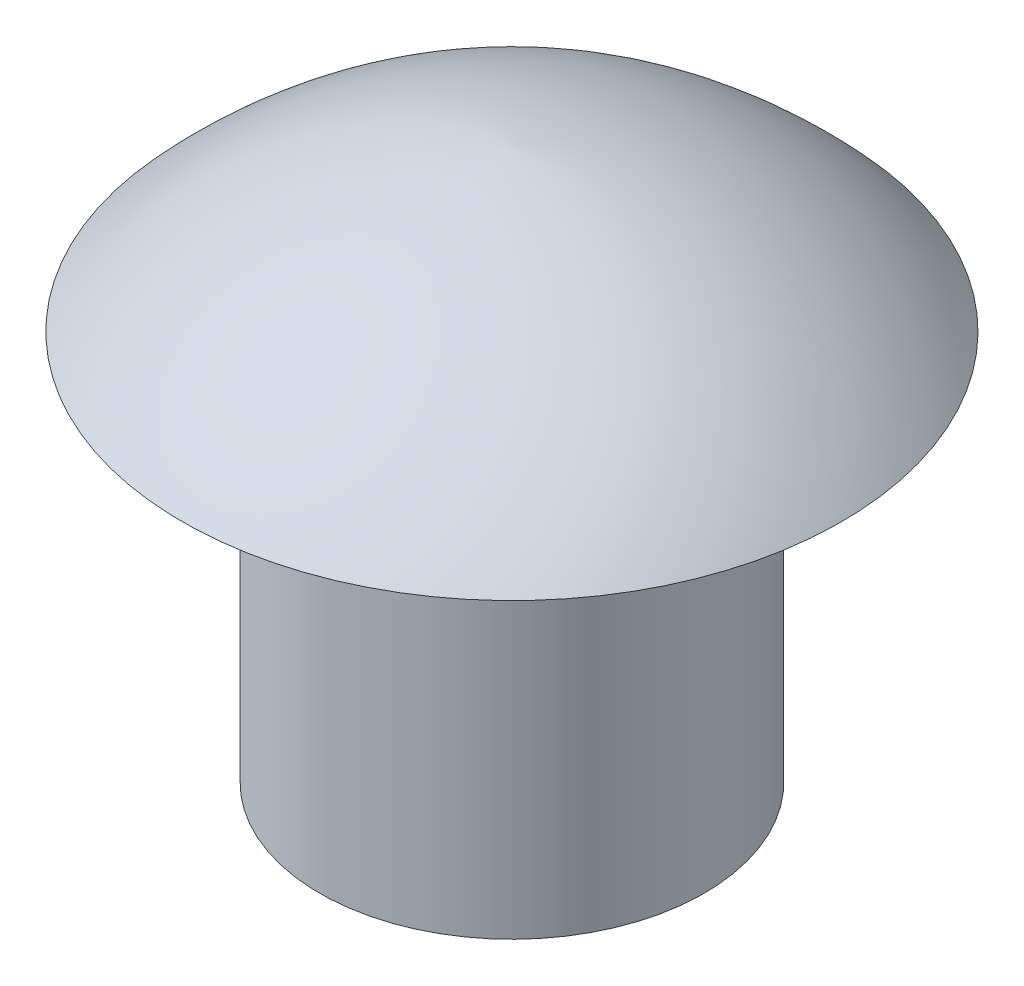
ISO-10303-21;
HEADER;
FILE_DESCRIPTION(('STEP AP214'),'2;1');
FILE_NAME('part.step','',(''),(''),'','','');
FILE_SCHEMA(('AUTOMOTIVE_DESIGN { 1 0 10303 214 1 1 1 1 }'));
ENDSEC;
DATA;
#1=APPLICATION_CONTEXT('core data for automotive mechanical design processes');
#2=APPLICATION_PROTOCOL_DEFINITION('international standard','automotive_design',2000,#1);
#3=PRODUCT_CONTEXT('',#1,'mechanical');
#4=PRODUCT('Part','Part','',(#3));
#5=PRODUCT_RELATED_PRODUCT_CATEGORY('part','',(#4));
#6=PRODUCT_DEFINITION_FORMATION('','',#4);
#7=PRODUCT_DEFINITION_CONTEXT('part definition',#1,'design');
#8=PRODUCT_DEFINITION('design','',#6,#7);
#9=PRODUCT_DEFINITION_SHAPE('','',#8);
#10=(LENGTH_UNIT() NAMED_UNIT(*) SI_UNIT(.MILLI.,.METRE.));
#11=(NAMED_UNIT(*) PLANE_ANGLE_UNIT() SI_UNIT($,.RADIAN.));
#12=(NAMED_UNIT(*) SI_UNIT($,.STERADIAN.) SOLID_ANGLE_UNIT());
#13=UNCERTAINTY_MEASURE_WITH_UNIT(LENGTH_MEASURE(1.E-05),#10,'distance_accuracy_value','');
#14=(GEOMETRIC_REPRESENTATION_CONTEXT(3) GLOBAL_UNCERTAINTY_ASSIGNED_CONTEXT((#13)) GLOBAL_UNIT_ASSIGNED_CONTEXT((#10,
#11,#12)) REPRESENTATION_CONTEXT('',''));
#15=CARTESIAN_POINT('',(0.,0.,0.));
#16=DIRECTION('',(0.,0.,1.));
#17=DIRECTION('',(1.,0.,0.));
#18=AXIS2_PLACEMENT_3D('',#15,#16,#17);
#19=CARTESIAN_POINT('',(0.,0.,0.));
#20=DIRECTION('',(0.,-1.,0.));
#21=DIRECTION('',(0.,0.,-1.));
#22=AXIS2_PLACEMENT_3D('',#19,#20,#21);
#23=PLANE('',#22);
#24=CARTESIAN_POINT('',(0.,0.,0.));
#25=DIRECTION('',(0.,-1.,0.));
#26=DIRECTION('',(0.,0.,-1.));
#27=AXIS2_PLACEMENT_3D('',#24,#25,#26);
#28=CIRCLE('',#27,1.75);
#29=CARTESIAN_POINT('',(0.,0.,-1.75));
#30=VERTEX_POINT('',#29);
#31=EDGE_CURVE('E11',#30,#30,#28,.T.);
#32=ORIENTED_EDGE('',*,*,#31,.T.);
#33=EDGE_LOOP('',(#32));
#34=FACE_BOUND('',#33,.T.);
#35=ADVANCED_FACE('F39',(#34),#23,.T.);
#36=CARTESIAN_POINT('',(0.,0.,0.));
#37=DIRECTION('',(0.,-1.,0.));
#38=DIRECTION('',(0.,0.,-1.));
#39=AXIS2_PLACEMENT_3D('',#36,#37,#38);
#40=CYLINDRICAL_SURFACE('',#39,1.75);
#41=CARTESIAN_POINT('',(0.,3.55388259495114,0.));
#42=DIRECTION('',(0.,-1.,0.));
#43=DIRECTION('',(0.,0.,-1.));
#44=AXIS2_PLACEMENT_3D('',#41,#42,#43);
#45=CIRCLE('',#44,1.75);
#46=CARTESIAN_POINT('',(0.,3.55388259495114,-1.75));
#47=VERTEX_POINT('',#46);
#48=EDGE_CURVE('E44',#47,#47,#45,.T.);
#49=ORIENTED_EDGE('',*,*,#48,.T.);
#50=EDGE_LOOP('',(#49));
#51=FACE_BOUND('',#50,.T.);
#52=ORIENTED_EDGE('',*,*,#31,.F.);
#53=EDGE_LOOP('',(#52));
#54=FACE_BOUND('',#53,.T.);
#55=ADVANCED_FACE('F62',(#51,#54),#40,.T.);
#56=CARTESIAN_POINT('',(1.75,3.55388259495114,0.));
#57=DIRECTION('',(0.,-1.,0.));
#58=DIRECTION('',(0.,0.,-1.));
#59=AXIS2_PLACEMENT_3D('',#56,#57,#58);
#60=PLANE('',#59);
#61=CARTESIAN_POINT('',(0.,3.55388259495114,0.));
#62=DIRECTION('',(0.,-1.,0.));
#63=DIRECTION('',(0.,0.,-1.));
#64=AXIS2_PLACEMENT_3D('',#61,#62,#63);
#65=CIRCLE('',#64,3.);
#66=CARTESIAN_POINT('',(0.,3.55388259495114,-3.));
#67=VERTEX_POINT('',#66);
#68=EDGE_CURVE('E54',#67,#67,#65,.T.);
#69=ORIENTED_EDGE('',*,*,#68,.T.);
#70=EDGE_LOOP('',(#69));
#71=FACE_BOUND('',#70,.T.);
#72=ORIENTED_EDGE('',*,*,#48,.F.);
#73=EDGE_LOOP('',(#72));
#74=FACE_BOUND('',#73,.T.);
#75=ADVANCED_FACE('F51',(#71,#74),#60,.T.);
#76=CARTESIAN_POINT('',(0.,0.511059760578535,0.315302278619654));
#77=DIRECTION('',(-1.,0.,0.));
#78=DIRECTION('',(0.,0.,-1.));
#79=AXIS2_PLACEMENT_3D('',#76,#77,#78);
#80=CIRCLE('',#79,4.5);
#81=TRIMMED_CURVE('',#80,(PARAMETER_VALUE(-1.5006716953399)),(PARAMETER_VALUE(1.5006716953399)),
.T.,.PARAMETER.);
#82=CARTESIAN_POINT('',(0.,0.511059760578535,0.));
#83=DIRECTION('',(0.,-1.,0.));
#84=AXIS1_PLACEMENT('',#82,#83);
#85=SURFACE_OF_REVOLUTION('',#81,#84);
#86=CARTESIAN_POINT('',(0.,5.,0.));
#87=VERTEX_POINT('',#86);
#88=VERTEX_LOOP('',#87);
#89=FACE_BOUND('',#88,.T.);
#90=ORIENTED_EDGE('',*,*,#68,.F.);
#91=EDGE_LOOP('',(#90));
#92=FACE_BOUND('',#91,.T.);
#93=ADVANCED_FACE('F48',(#89,#92),#85,.T.);
#94=CLOSED_SHELL('',(#35,#55,#75,#93));
#95=MANIFOLD_SOLID_BREP('B2',#94);
#96=ADVANCED_BREP_SHAPE_REPRESENTATION('',(#18,#95),#14);
#97=SHAPE_DEFINITION_REPRESENTATION(#9,#96);
ENDSEC;
END-ISO-10303-21;
